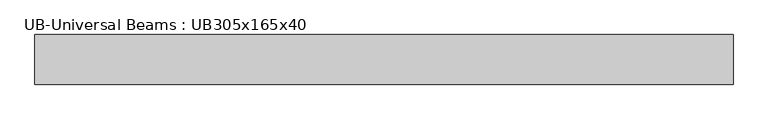
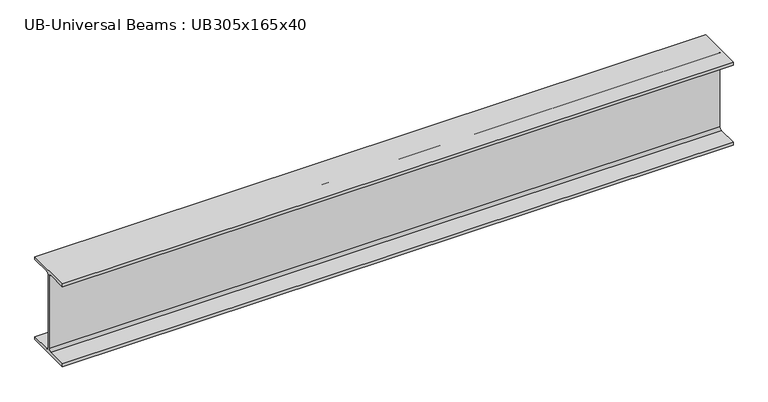
"""IFC4 building model written with IfcOpenShell, lengths in millimetres: beam geometry, UB-Universal Beams : UB305x165x40."""

from ifc_helpers import new_model, si_unit, point, frame, frame_2d, origin, place, context, project, spatial, polyline, circle_curve, trimmed, segment, composite_curve, outline, extrude, source, transform, mapped, element, save


def ub_universal_beams_ub305x165x40_9aefeb6a(model_context):
    return source(origin(), model_context, "Body", "SweptSolid", [
        extrude(outline(composite_curve([segment(polyline([(82.5, -141.5), (82.5, -151.7), (-82.5, -151.7), (-82.5, -141.5), (-11.9, -141.5)]), True, "CONTINUOUS"), segment(trimmed(circle_curve(frame_2d((-11.9, -132.6)), 8.9), [point((-11.9, -141.5))], [point((-3.0, -132.6))], True, "CARTESIAN"), True, "CONTINUOUS"), segment(polyline([(-3.0, -132.6), (-3.0, 132.6)]), True, "CONTINUOUS"), segment(trimmed(circle_curve(frame_2d((-11.9, 132.6)), 8.9), [point((-3.0, 132.6))], [point((-11.9, 141.5))], True, "CARTESIAN"), True, "CONTINUOUS"), segment(polyline([(-11.9, 141.5), (-82.5, 141.5), (-82.5, 151.7), (82.5, 151.7), (82.5, 141.5), (11.9, 141.5)]), True, "CONTINUOUS"), segment(trimmed(circle_curve(frame_2d((11.9, 132.6)), 8.9), [point((11.9, 141.5))], [point((3.0, 132.6))], True, "CARTESIAN"), True, "CONTINUOUS"), segment(polyline([(3.0, 132.6), (3.0, -132.6)]), True, "CONTINUOUS"), segment(trimmed(circle_curve(frame_2d((11.9, -132.6)), 8.9), [point((3.0, -132.6))], [point((11.9, -141.5))], True, "CARTESIAN"), True, "CONTINUOUS"), segment(polyline([(11.9, -141.5), (82.5, -141.5)]), True, "CONTINUOUS")], self_intersect=False)), frame((-1229.9, 0.0, 0.0), z_axis=(1.0, 0.0, 0.0), x_axis=(0.0, 1.0, 0.0)), (0.0, 0.0, 1.0), 2323.0),
    ])


if __name__ == "__main__":
    model = new_model("IFC4")
    model_context = context("Model", 3, world=origin())
    ifc_project = project(units=[si_unit("LENGTHUNIT", "METRE", prefix="MILLI")], contexts=[model_context])
    site = spatial("IfcSite", under=ifc_project)
    building = spatial("IfcBuilding", under=site)
    placement = place(None, origin())
    ub_universal_beams_ub305x165x40_shape = ub_universal_beams_ub305x165x40_9aefeb6a(model_context)
    element("IfcBeam", 1, ObjectType="UB-Universal Beams : UB305x165x40", at=placement, inside=building, context=model_context, shape_type="MappedRepresentation", body=[
        mapped(ub_universal_beams_ub305x165x40_shape, transform((0.0, 0.0, 0.0), x_axis=(1.0, 0.0, 0.0), y_axis=(0.0, 1.0, 0.0), z_axis=(0.0, 0.0, 1.0))),
    ])
    save(model, "model.ifc")

# Revit data of these elements
# Type "UB-Universal Beams : UB305x165x40"
#   Section Name Key = "UB305X165X40"
#   Width = 16.5 cm
#   Web Thickness = 0.6 cm
#   Web Fillet = 0.89 cm
#   Warping Constant = 164000.0 cm⁶
#   Torsional Moment of Inertia = 14.70 cm⁴
#   Section Area = 51.3 cm²
#   Plastic Modulus weak axis = 142.0 cm³
#   Plastic Modulus strong axis = 623.0 cm³
#   Nominal Weight = 40.2999 kgf/m
#   Moment of Inertia weak axis = 764.00 cm⁴
#   Moment of Inertia strong axis = 8503.00 cm⁴
#   Height = 30.34 cm
#   Flange Thickness = 1.02 cm
#   Elastic Modulus weak axis = 92.6 cm³
#   Elastic Modulus strong axis = 560.0 cm³
#   Centroid Vertical = 15.17 cm
#   Centroid Horizontal = 8.25 cm
#   Bolt Spacing = 9.0 cm
#   Length [instance default] = 1500 mm
#   Structural Material [instance default] = Metal - Steel 43-275
#   Type Comments = ""
#   Assembly Code = ""
# Element 1 (IfcBeam, "UB-Universal Beams : UB305x165x40")
#   Materials on its faces: "Metal - Steel 43-275"
# Materials
#   "Metal - Steel 43-275": class "Metal", colour RGB 247 247 247, transparency 0, Cost = 0
